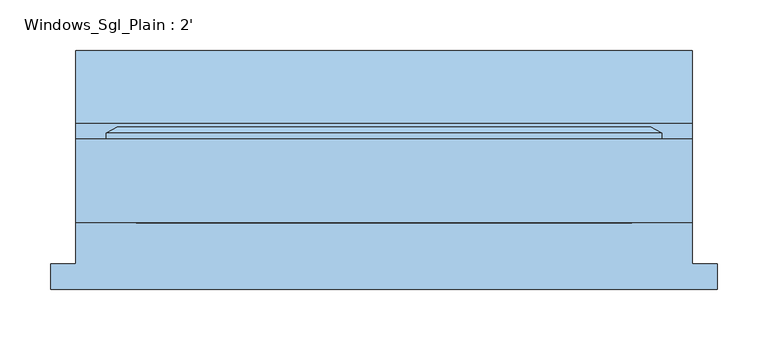
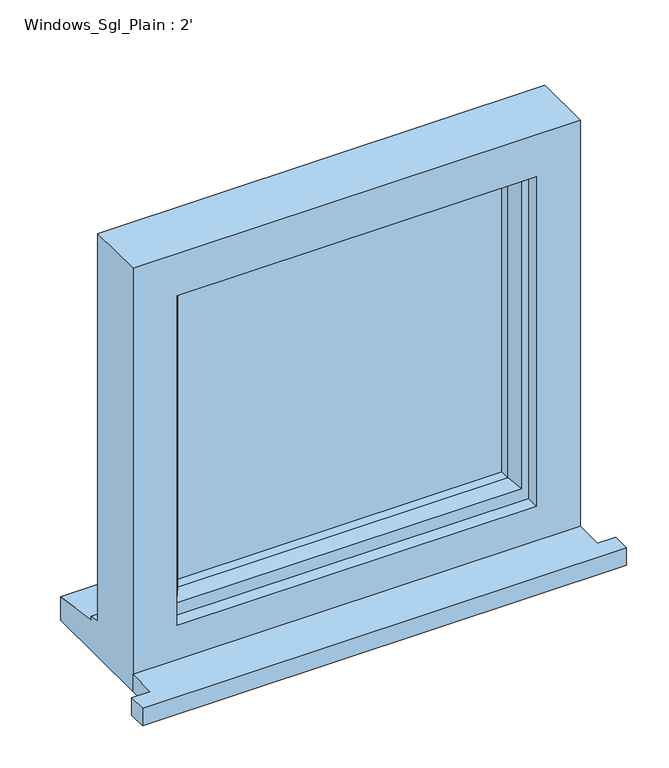
"""IFC4 building model written with IfcOpenShell, lengths in millimetres: window geometry, Windows_Sgl_Plain : 2'."""

from ifc_helpers import new_model, si_unit, frame, origin, place, context, project, spatial, polyline, outline, extrude, faceted_brep, source, transform, mapped, element, save


def windows_sgl_plain_2_43817c1b(model_context):
    return source(origin(), model_context, "Body", "SolidModel", [
        extrude(outline(polyline([(-329.8, -103.4114322), (-329.8, -78.4114322), (-304.8, -78.4114322), (-304.8, -37.6754322), (304.8, -37.6754322), (304.8, -78.4114322), (329.8, -78.4114322), (329.8, -103.4114322), (-329.8, -103.4114322)])), frame((0.0, 0.0, 1500.4), z_axis=(0.0, 0.0, 1.0), x_axis=(1.0, 0.0, 0.0)), (0.0, 0.0, 1.0), 25.0),
        faceted_brep([(-304.8, -37.6754322, 1500.4), (304.8, -37.6754322, 1500.4), (304.8, -37.6754322, 2110.0), (-304.8, -37.6754322, 2110.0), (-244.8, -37.6754322, 2050.0), (244.8, -37.6754322, 2050.0), (244.8, -37.6754322, 1575.4), (-244.8, -37.6754322, 1575.4), (-304.8, 45.3245678, 2110.0), (-304.8, 45.3245678, 1551.4), (-304.8, 60.3245678, 1550.08767), (-304.8, 60.3245678, 1545.1449676), (-304.8, 132.8245678, 1534.2088847), (-304.8, 132.8245678, 1500.4), (304.8, 45.3245678, 2110.0), (304.8, 45.3245678, 1551.4), (-264.8, 45.3245678, 2070.0), (-264.8, 45.3245678, 1563.4), (264.8, 45.3245678, 1563.4), (264.8, 45.3245678, 2070.0), (-264.8, -19.6754322, 2070.0), (-264.8, -19.6754322, 1563.4), (264.8, -19.6754322, 2070.0), (264.8, -19.6754322, 1563.4), (-244.8, -19.6754322, 2050.0), (-244.8, -19.6754322, 1575.4), (244.8, -19.6754322, 1575.4), (244.8, -19.6754322, 2050.0), (304.8, 132.8245678, 1500.4), (304.8, 132.8245678, 1534.2088847), (304.8, 60.3245678, 1545.1449676), (304.8, 60.3245678, 1550.08767)], [[[0, 1, 2, 3], [4, 5, 6, 7]], [[0, 3, 8, 9, 10, 11, 12, 13]], [[9, 8, 14, 15], [16, 17, 18, 19]], [[17, 16, 20, 21]], [[20, 22, 23, 21], [24, 25, 26, 27]], [[24, 4, 7, 25]], [[3, 2, 14, 8]], [[16, 19, 22, 20]], [[5, 4, 24, 27]], [[15, 14, 2, 1, 28, 29, 30, 31]], [[19, 18, 23, 22]], [[5, 27, 26, 6]], [[28, 1, 0, 13]], [[29, 28, 13, 12]], [[30, 29, 12, 11]], [[31, 30, 11, 10]], [[15, 31, 10, 9]], [[21, 23, 18, 17]], [[7, 6, 26, 25]]]),
        extrude(outline(polyline([(234.8, 9.3245678), (-234.8, 9.3245678), (-234.8, 33.3245678), (234.8, 33.3245678), (234.8, 9.3245678)])), frame((0.0, 0.0, 1593.4), z_axis=(0.0, 0.0, 1.0), x_axis=(1.0, 0.0, 0.0)), (0.0, 0.0, 1.0), 446.6),
        faceted_brep([(-274.8, 45.3245678, 2080.0), (-274.8, 51.0980705, 2080.0), (-274.8, 51.0980705, 1553.4), (-274.8, 45.3245678, 1553.4), (-264.8, -19.6754322, 2070.0), (-264.8, 45.3245678, 2070.0), (-264.8, 45.3245678, 1563.4), (-264.8, -19.6754322, 1563.4), (-224.8, -5.1825323, 2030.0), (-234.9480377, -19.6754322, 2040.1480377), (-234.9480377, -19.6754322, 1593.2519623), (-224.8, -5.1825323, 1603.4), (-224.8, 9.3245678, 2030.0), (-224.8, 9.3245678, 1603.4), (-234.8, 33.3245678, 2040.0), (-234.8, 9.3245678, 2040.0), (-234.8, 9.3245678, 1593.4), (-234.8, 33.3245678, 1593.4), (-224.8, 51.0980705, 2030.0), (-224.8, 33.3245678, 2030.0), (-224.8, 33.3245678, 1603.4), (-224.8, 51.0980705, 1603.4), (-242.2457548, 56.8715732, 2047.4457548), (-242.2457548, 56.8715732, 1585.9542452), (-264.0153903, 56.8715732, 2069.2153903), (-264.0153903, 56.8715732, 1564.1846097), (274.8, 51.0980705, 1553.4), (274.8, 45.3245678, 1553.4), (264.8, 45.3245678, 1563.4), (264.8, -19.6754322, 1563.4), (234.9480377, -19.6754322, 1593.2519623), (224.8, -5.1825323, 1603.4), (224.8, 9.3245678, 1603.4), (234.8, 9.3245678, 1593.4), (234.8, 33.3245678, 1593.4), (224.8, 33.3245678, 1603.4), (224.8, 51.0980705, 1603.4), (242.2457548, 56.8715732, 1585.9542452), (264.0153903, 56.8715732, 1564.1846097), (274.8, 51.0980705, 2080.0), (274.8, 45.3245678, 2080.0), (264.8, 45.3245678, 2070.0), (264.8, -19.6754322, 2070.0), (234.9480377, -19.6754322, 2040.1480377), (224.8, -5.1825323, 2030.0), (224.8, 9.3245678, 2030.0), (234.8, 9.3245678, 2040.0), (234.8, 33.3245678, 2040.0), (224.8, 33.3245678, 2030.0), (224.8, 51.0980705, 2030.0), (242.2457548, 56.8715732, 2047.4457548), (264.0153903, 56.8715732, 2069.2153903)], [[[0, 1, 2, 3]], [[4, 5, 6, 7]], [[8, 9, 10, 11]], [[12, 8, 11, 13]], [[14, 15, 16, 17]], [[18, 19, 20, 21]], [[22, 18, 21, 23]], [[1, 24, 25, 2]], [[3, 2, 26, 27]], [[7, 6, 28, 29]], [[11, 10, 30, 31]], [[13, 11, 31, 32]], [[17, 16, 33, 34]], [[21, 20, 35, 36]], [[23, 21, 36, 37]], [[2, 25, 38, 26]], [[27, 26, 39, 40]], [[29, 28, 41, 42]], [[31, 30, 43, 44]], [[32, 31, 44, 45]], [[34, 33, 46, 47]], [[36, 35, 48, 49]], [[37, 36, 49, 50]], [[26, 38, 51, 39]], [[40, 39, 1, 0]], [[3, 27, 40, 0], [5, 41, 28, 6]], [[42, 41, 5, 4]], [[7, 29, 42, 4], [9, 43, 30, 10]], [[44, 43, 9, 8]], [[45, 44, 8, 12]], [[15, 46, 33, 16], [13, 32, 45, 12]], [[47, 46, 15, 14]], [[17, 34, 47, 14], [19, 48, 35, 20]], [[49, 48, 19, 18]], [[50, 49, 18, 22]], [[24, 51, 38, 25], [23, 37, 50, 22]], [[39, 51, 24, 1]]]),
    ])


if __name__ == "__main__":
    model = new_model("IFC4")
    model_context = context("Model", 3, world=origin())
    ifc_project = project(units=[si_unit("LENGTHUNIT", "METRE", prefix="MILLI")], contexts=[model_context])
    site = spatial("IfcSite", under=ifc_project)
    building = spatial("IfcBuilding", under=site)
    placement = place(None, origin())
    windows_sgl_plain_2_shape = windows_sgl_plain_2_43817c1b(model_context)
    element("IfcWindow", 1, ObjectType="Windows_Sgl_Plain : 2'", at=placement, inside=building, context=model_context, shape_type="MappedRepresentation", body=[
        mapped(windows_sgl_plain_2_shape, transform((0.0, 0.0, 0.0), x_axis=(1.0, 0.0, 0.0), y_axis=(0.0, 1.0, 0.0), z_axis=(0.0, 0.0, 1.0))),
    ])
    save(model, "model.ifc")

# Revit data of these elements
# Type "Windows_Sgl_Plain : 2'"
#   Type Mark = "60"
#   Operation = "SinglePanel"
#   Construction Type Id = "SGL"
#   Manufacturer = "Revit"
#   Keynote = "L10"
#   Analytic Construction = "Large single-glazed windows"
#   Wrap Layers (Ext) from Ext = 0.336286 ft
#   Wrap Layers (Int) from Ext = 0.582349 ft
#   Window Board Projection = 0.082021 ft
#   Window Board Extension = 0.082021 ft
#   Visual Light Transmittance = 0.9
#   Solar Heat Gain Coefficient = 0.86
#   Rough Width = 2.0 ft
#   Rough Height = 2.0 ft
#   Height = 2.0 ft
#   Width = 2.0 ft
#   Heat Transfer Coefficient (U) = 5.5617 W/(m²·K)
#   Glazing Thickness = 0.07874 ft
#   FrameOffset - External = 0.164042 ft
#   Frame Depth = 0.213255 ft
#   Default Head Height = 6.922572 ft
#   Cill Depth = 0.287073 ft
#   Cavity Closer Width = 0.164042 ft
#   Cavity Closer Offset from Ext = 0.336286 ft
#   Cavity Closer Depth = 0.278871 ft
#   Vis - Cavity Closers = yes
#   Define Thermal Properties by = 1
#   Material Trim = Window Frame
#   Material Glass = Glass
#   Material Frame = Window Frame
#   Wall Closure = (empty or 0)
# Element 1 (IfcWindow, "Windows_Sgl_Plain : 2'")
#   Materials on its faces: "Window Frame", "Glass"
# Materials
#   "Window Frame": colour RGB 249 249 249, transparency 0, Keynote = "L10", Cost = 0
#   "Glass": class "Glass", colour RGB 0 128 192, transparency 0.9, Description = "Soda Lime Glass", Cost = 0
